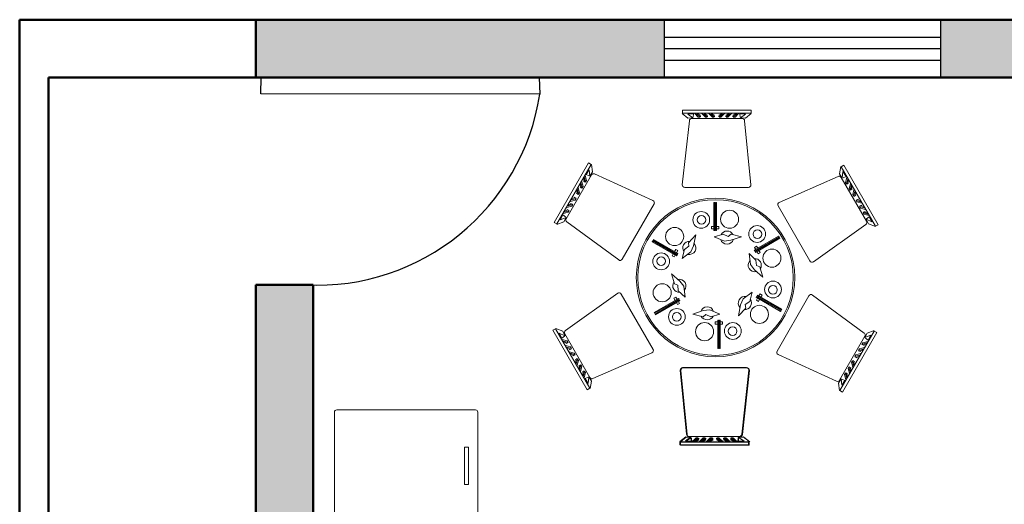
# Model space of a CAD drawing. Units: inches. Extents: x 1771 to 3025, y 319 to 889.
# Tile 32 of 35: x 2683 to 2854, y 805 to 889. Entities that reach past the tile are written whole.
import ezdxf

# ---------------------------------------------------------------- set-up
doc = ezdxf.new("R2010")
doc.units = ezdxf.units.IN
doc.header["$MEASUREMENT"] = 0
for name, color, linetype, lineweight in [('A-DOOR', 4, 'Continuous', 25), ('A-FURN', 8, 'Continuous', 18), ('A-GLAZ', 40, 'Continuous', 25), ('A-WALL', 7, 'Continuous', 50), ('A-WALL-PATT', 254, 'Continuous', 13)]:
    doc.layers.add(name, color=color, linetype=linetype, lineweight=lineweight)

# ---------------------------------------------------------------- blocks, each defined once
blk = doc.blocks.new('A$C1C317F9A')
for p, q in [((0.8756, 2.2462), (0.9155, 2.2143)), ((0.8788, 2.2685), (0.8788, 2.2478)), ((1.3449, 2.2685), (0.8788, 2.2685)), ((0.8788, 2.2478), (1.3449, 2.2478)), ((0.9139, 2.2414), (0.9522, 2.243)), ((0.949, 2.2159), (0.9139, 2.2414)), ((0.9155, 2.2143), (0.949, 2.2159)), ((0.941, 2.2111), (1.2841, 2.2111)), ((0.9522, 2.243), (0.9506, 2.2206)), ((0.9618, 2.2446), (0.9857, 2.2206)), ((0.9745, 2.243), (0.9841, 2.243)), ((0.9985, 2.2206), (0.9745, 2.243)), ((0.9841, 2.243), (0.9953, 2.2334)), ((0.9857, 2.2206), (0.9985, 2.2206)), ((0.9953, 2.2334), (0.9985, 2.2366)), ((0.9985, 2.2366), (1.0001, 2.2222)), ((1.0097, 2.2446), (1.0336, 2.2206)), ((1.0224, 2.243), (1.032, 2.243)), ((1.0464, 2.2206), (1.0224, 2.243)), ((1.032, 2.243), (1.0432, 2.2334)), ((1.0336, 2.2206), (1.0464, 2.2206)), ((1.0432, 2.2334), (1.0464, 2.2366)), ((1.0464, 2.2366), (1.048, 2.2222)), ((1.0576, 2.2446), (1.0815, 2.2206)), ((1.0703, 2.243), (1.0799, 2.243)), ((1.0943, 2.2206), (1.0703, 2.243)), ((1.0799, 2.243), (1.0911, 2.2334)), ((1.0815, 2.2206), (1.0943, 2.2206)), ((1.0911, 2.2334), (1.0943, 2.2366)), ((1.0943, 2.2366), (1.0959, 2.2222)), ((1.1262, 2.2366), (1.1246, 2.2222)), ((1.1262, 2.2206), (1.1502, 2.243)), ((1.1294, 2.2334), (1.1262, 2.2366)), ((1.139, 2.2206), (1.1262, 2.2206)), ((1.1406, 2.243), (1.1294, 2.2334)), ((1.1629, 2.2446), (1.139, 2.2206)), ((1.1502, 2.243), (1.1406, 2.243)), ((1.1741, 2.2366), (1.1725, 2.2222)), ((1.1741, 2.2206), (1.1981, 2.243)), ((1.1773, 2.2334), (1.1741, 2.2366)), ((1.1869, 2.2206), (1.1741, 2.2206)), ((1.1885, 2.243), (1.1773, 2.2334)), ((1.2108, 2.2446), (1.1869, 2.2206)), ((1.1981, 2.243), (1.1885, 2.243)), ((1.222, 2.2366), (1.2204, 2.2222)), ((1.222, 2.2206), (1.246, 2.243)), ((1.2252, 2.2334), (1.222, 2.2366)), ((1.2348, 2.2206), (1.222, 2.2206)), ((1.2364, 2.243), (1.2252, 2.2334)), ((1.2587, 2.2446), (1.2348, 2.2206)), ((1.246, 2.243), (1.2364, 2.243)), ((1.2683, 2.243), (1.2699, 2.2206)), ((1.3066, 2.2414), (1.2683, 2.243)), ((1.2715, 2.2159), (1.3066, 2.2414)), ((1.305, 2.2143), (1.2715, 2.2159)), ((1.3449, 2.2462), (1.305, 2.2143)), ((1.3449, 2.2478), (1.3449, 2.2685)), ((0.8775, 1.7628), (0.9251, 2.1968)), ((1.3, 2.1966), (1.3417, 1.7626)), ((0.2422, 1.9115), (0.0091, 1.5078)), ((0.0271, 1.4974), (0.2602, 1.9011)), ((0.2602, 1.9011), (0.2422, 1.9115)), ((0.2615, 1.9003), (0.2692, 1.8498)), ((1.9514, 1.8873), (1.9438, 1.8368)), ((1.9724, 1.8957), (1.9544, 1.8854)), ((1.9544, 1.8854), (2.1875, 1.4816)), ((2.2055, 1.492), (1.9724, 1.8957)), ((0.09, 1.5329), (0.2615, 1.8301)), ((0.2148, 1.813), (0.21, 1.8047)), ((0.21, 1.8047), (0.2127, 1.7903)), ((0.2222, 1.7811), (0.2148, 1.813)), ((0.2198, 1.8249), (0.2286, 1.7922)), ((0.2465, 1.8648), (0.226, 1.8324)), ((0.226, 1.8324), (0.2461, 1.8226)), ((0.2511, 1.8216), (0.2465, 1.8648)), ((0.2692, 1.8498), (0.2511, 1.8216)), ((0.282, 1.8367), (0.6787, 1.6557)), ((1.5338, 1.644), (1.9335, 1.8198)), ((1.9438, 1.8368), (1.9619, 1.8086)), ((1.9537, 1.8131), (2.1253, 1.516)), ((1.9619, 1.8086), (1.9665, 1.8518)), ((1.9665, 1.8518), (1.987, 1.8194)), ((1.987, 1.8194), (1.9669, 1.8096)), ((1.9932, 1.8119), (1.9844, 1.7792)), ((0.1719, 1.7419), (0.1807, 1.7092)), ((0.1888, 1.7488), (0.1844, 1.7476)), ((0.1844, 1.7476), (0.1961, 1.7391)), ((0.1909, 1.7716), (0.1861, 1.7633)), ((0.1861, 1.7633), (0.1888, 1.7488)), ((0.1982, 1.7396), (0.1909, 1.7716)), ((0.1959, 1.7834), (0.2046, 1.7507)), ((0.2046, 1.7507), (0.1982, 1.7396)), ((0.2127, 1.7903), (0.2084, 1.7891)), ((0.2084, 1.7891), (0.22, 1.7805)), ((0.2286, 1.7922), (0.2222, 1.7811)), ((1.3258, 1.7451), (0.8934, 1.7451)), ((1.9844, 1.7792), (1.9908, 1.7681)), ((1.9908, 1.7681), (1.9982, 1.8)), ((2.0046, 1.7761), (1.993, 1.7675)), ((1.9982, 1.8), (2.003, 1.7917)), ((2.003, 1.7917), (2.0003, 1.7773)), ((2.0003, 1.7773), (2.0046, 1.7761)), ((2.0171, 1.7704), (2.0084, 1.7377)), ((2.0084, 1.7377), (2.0147, 1.7266)), ((2.0147, 1.7266), (2.0221, 1.7585)), ((2.0221, 1.7585), (2.0269, 1.7502)), ((2.0269, 1.7502), (2.0242, 1.7358)), ((2.0242, 1.7358), (2.0286, 1.7346)), ((0.1583, 1.6705), (0.127, 1.6609)), ((0.127, 1.6609), (0.1318, 1.6692)), ((0.1318, 1.6692), (0.1457, 1.6741)), ((0.1445, 1.6785), (0.1577, 1.6727)), ((0.1457, 1.6741), (0.1445, 1.6785)), ((0.1519, 1.6595), (0.1583, 1.6705)), ((0.1648, 1.7073), (0.1605, 1.7061)), ((0.1605, 1.7061), (0.1721, 1.6976)), ((0.1669, 1.7301), (0.1621, 1.7218)), ((0.1621, 1.7218), (0.1648, 1.7073)), ((0.1743, 1.6982), (0.1669, 1.7301)), ((0.1807, 1.7092), (0.1743, 1.6982)), ((2.0286, 1.7346), (2.0169, 1.726)), ((2.0411, 1.7289), (2.0323, 1.6962)), ((2.0323, 1.6962), (2.0387, 1.6852)), ((2.0387, 1.6852), (2.0461, 1.7171)), ((2.0525, 1.6931), (2.0409, 1.6846)), ((2.0461, 1.7171), (2.0509, 1.7088)), ((2.0509, 1.7088), (2.0482, 1.6943)), ((2.0482, 1.6943), (2.0525, 1.6931)), ((0.0953, 1.6092), (0.128, 1.618)), ((0.1344, 1.629), (0.1031, 1.6195)), ((0.1031, 1.6195), (0.1078, 1.6278)), ((0.1078, 1.6278), (0.1217, 1.6327)), ((0.1192, 1.6507), (0.1519, 1.6595)), ((0.1217, 1.6327), (0.1206, 1.637)), ((0.1206, 1.637), (0.1338, 1.6312)), ((0.128, 1.618), (0.1344, 1.629)), ((0.6859, 1.6332), (0.4697, 1.2588)), ((1.091, 1.6437, 0.0908), (1.091, 1.4528, 0.0908)), ((1.097, 1.6437, 0.0908), (1.091, 1.6437, 0.0908)), ((1.097, 1.4528, 0.0908), (1.097, 1.6437, 0.0908)), ((1.1023, 1.6437, 0.0908), (1.1023, 1.4528, 0.0908)), ((1.1083, 1.6437, 0.0908), (1.1023, 1.6437, 0.0908)), ((1.1083, 1.4528, 0.0908), (1.1083, 1.6437, 0.0908)), ((1.7426, 1.2469), (1.5264, 1.6214)), ((2.0547, 1.6575), (2.086, 1.6479)), ((2.061, 1.6464), (2.0547, 1.6575)), ((2.0685, 1.6655), (2.0552, 1.6597)), ((2.0937, 1.6377), (2.061, 1.6464)), ((2.0673, 1.6611), (2.0685, 1.6655)), ((2.0812, 1.6562), (2.0673, 1.6611)), ((2.0786, 1.616), (2.1099, 1.6065)), ((2.085, 1.605), (2.0786, 1.616)), ((2.0924, 1.624), (2.0792, 1.6182)), ((2.086, 1.6479), (2.0812, 1.6562)), ((2.1177, 1.5962), (2.085, 1.605)), ((2.0913, 1.6196), (2.0924, 1.624)), ((2.1051, 1.6148), (2.0913, 1.6196)), ((2.1099, 1.6065), (2.1051, 1.6148)), ((0.0502, 1.5246), (0.0679, 1.5586)), ((0.0898, 1.5423), (0.0502, 1.5246)), ((0.0679, 1.5586), (0.0865, 1.5461)), ((0.0713, 1.5677), (0.104, 1.5765)), ((0.0745, 1.5125), (0.0898, 1.5423)), ((0.1104, 1.5876), (0.0791, 1.578)), ((0.0791, 1.578), (0.0839, 1.5863)), ((0.0839, 1.5863), (0.0978, 1.5912)), ((0.0966, 1.5955), (0.1098, 1.5897)), ((0.0978, 1.5912), (0.0966, 1.5955)), ((0.104, 1.5765), (0.1104, 1.5876)), ((2.1026, 1.5745), (2.1339, 1.565)), ((2.1089, 1.5635), (2.1026, 1.5745)), ((2.1164, 1.5825), (2.1031, 1.5767)), ((2.1416, 1.5547), (2.1089, 1.5635)), ((2.1152, 1.5782), (2.1164, 1.5825)), ((2.1291, 1.5733), (2.1152, 1.5782)), ((2.145, 1.5456), (2.1265, 1.5331)), ((2.1339, 1.565), (2.1291, 1.5733)), ((2.1628, 1.5116), (2.145, 1.5456)), ((0.0091, 1.5078), (0.0271, 1.4974)), ((0.0269, 1.4939), (0.0745, 1.5125)), ((0.4464, 1.2539), (0.0943, 1.5121)), ((1.0755, 1.4796, 0.0908), (1.0755, 1.4641, 0.0908)), ((1.091, 1.4796, 0.0908), (1.0755, 1.4796, 0.0908)), ((1.1023, 1.4796, 0.0908), (1.097, 1.4796, 0.0908)), ((1.125, 1.4796, 0.0908), (1.1083, 1.4796, 0.0908)), ((1.125, 1.4641, 0.0908), (1.125, 1.4796, 0.0908)), ((2.1208, 1.495), (1.7657, 1.2419)), ((2.1232, 1.5293), (2.1628, 1.5116)), ((2.1385, 1.4995), (2.1232, 1.5293)), ((2.1861, 1.4809), (2.1385, 1.4995)), ((2.1875, 1.4816), (2.2055, 1.492)), ((0.9684, 1.4231, 0.0908), (0.9184, 1.3706, 0.0908)), ((0.953, 1.3489, 0.0908), (0.9684, 1.4231, 0.0908)), ((1.0755, 1.4641, 0.0908), (1.091, 1.4641, 0.0908)), ((1.091, 1.4528, 0.0908), (1.097, 1.4528, 0.0908)), ((1.1549, 1.429, 0.0908), (1.0933, 1.4112, 0.0908)), ((1.0933, 1.4112, 0.0908), (1.1623, 1.3815, 0.0908)), ((1.097, 1.4641, 0.0908), (1.1023, 1.4641, 0.0908)), ((1.1023, 1.4528, 0.0908), (1.1083, 1.4528, 0.0908)), ((1.1083, 1.4641, 0.0908), (1.125, 1.4641, 0.0908)), ((1.1882, 1.4134, 0.0908), (1.1549, 1.429, 0.0908)), ((1.2075, 1.4282, 0.0908), (1.1882, 1.4134, 0.0908)), ((1.2061, 1.3874, 0.0908), (1.278, 1.4112, 0.0908)), ((1.278, 1.4112, 0.0908), (1.2075, 1.4282, 0.0908)), ((1.5304, 1.4154, 0.0908), (1.365, 1.3199, 0.0908)), ((1.368, 1.3147, 0.0908), (1.5334, 1.4102, 0.0908)), ((1.5361, 1.4055, 0.0908), (1.3707, 1.3101, 0.0908)), ((1.5334, 1.4102, 0.0908), (1.5304, 1.4154, 0.0908)), ((1.539, 1.4004, 0.0908), (1.5361, 1.4055, 0.0908)), ((0.6765, 1.3825, 0.0908), (0.6735, 1.3774, 0.0908)), ((0.6735, 1.3774, 0.0908), (0.8389, 1.2819, 0.0908)), ((0.8419, 1.2871, 0.0908), (0.6765, 1.3825, 0.0908)), ((0.6822, 1.3924, 0.0908), (0.6792, 1.3872, 0.0908)), ((0.6792, 1.3872, 0.0908), (0.8446, 1.2917, 0.0908)), ((0.8476, 1.2969, 0.0908), (0.6822, 1.3924, 0.0908)), ((0.9216, 1.3464, 0.0908), (0.8914, 1.3253, 0.0908)), ((0.9184, 1.3706, 0.0908), (0.9216, 1.3464, 0.0908)), ((0.9363, 1.308, 0.0908), (0.953, 1.3489, 0.0908)), ((1.1623, 1.3815, 0.0908), (1.2061, 1.3874, 0.0908)), ((1.3805, 1.3467, 0.0908), (1.3671, 1.339, 0.0908)), ((1.3671, 1.339, 0.0908), (1.3748, 1.3255, 0.0908)), ((1.3737, 1.3049, 0.0908), (1.539, 1.4004, 0.0908)), ((1.3883, 1.3333, 0.0908), (1.3805, 1.3467, 0.0908)), ((0.8156, 1.2953, 0.0908), (0.8079, 1.2819, 0.0908)), ((0.8079, 1.2819, 0.0908), (0.8213, 1.2741, 0.0908)), ((0.8213, 1.3051, 0.0908), (0.8186, 1.3005, 0.0908)), ((0.8213, 1.2741, 0.0908), (0.8291, 1.2876, 0.0908)), ((0.8327, 1.3248, 0.0908), (0.8243, 1.3103, 0.0908)), ((0.8321, 1.2927, 0.0908), (0.8348, 1.2974, 0.0908)), ((0.8461, 1.317, 0.0908), (0.8327, 1.3248, 0.0908)), ((0.8377, 1.3025, 0.0908), (0.8461, 1.317, 0.0908)), ((0.8389, 1.2819, 0.0908), (0.8419, 1.2871, 0.0908)), ((0.8446, 1.2917, 0.0908), (0.8476, 1.2969, 0.0908)), ((0.8914, 1.3253, 0.0908), (0.8761, 1.2631, 0.0908)), ((0.8761, 1.2631, 0.0908), (0.9363, 1.308, 0.0908)), ((1.3763, 1.2527, 0.0908), (1.3301, 1.2971, 0.0908)), ((1.3301, 1.2971, 0.0908), (1.3389, 1.2225, 0.0908)), ((1.365, 1.3199, 0.0908), (1.368, 1.3147, 0.0908)), ((1.3707, 1.3101, 0.0908), (1.3737, 1.3049, 0.0908)), ((1.3778, 1.3204, 0.0908), (1.3805, 1.3157, 0.0908)), ((1.3835, 1.3106, 0.0908), (1.3918, 1.2961, 0.0908)), ((1.3939, 1.3235, 0.0908), (1.3912, 1.3281, 0.0908)), ((1.3918, 1.2961, 0.0908), (1.4053, 1.3038, 0.0908)), ((1.4053, 1.3038, 0.0908), (1.3969, 1.3183, 0.0908)), ((1.3389, 1.2225, 0.0908), (1.366, 1.1876, 0.0908)), ((1.3795, 1.216, 0.0908), (1.3763, 1.2527, 0.0908)), ((1.402, 1.2067, 0.0908), (1.3795, 1.216, 0.0908)), ((1.4225, 1.1371, 0.0908), (1.402, 1.2067, 0.0908)), ((0.8033, 1.1609, 0.0908), (0.8238, 1.0913, 0.0908)), ((0.8599, 1.1105, 0.0908), (0.8033, 1.1609, 0.0908)), ((1.366, 1.1876, 0.0908), (1.4225, 1.1371, 0.0908)), ((0.8238, 1.0913, 0.0908), (0.8463, 1.0821, 0.0908)), ((0.8463, 1.0821, 0.0908), (0.8495, 1.0454, 0.0908)), ((0.8869, 1.0755, 0.0908), (0.8599, 1.1105, 0.0908)), ((0.8957, 1.0009, 0.0908), (0.8869, 1.0755, 0.0908)), ((0.0847, 0.7751), (0.4398, 1.0281)), ((0.4628, 1.0231), (0.679, 0.6486)), ((0.834, 1.0019, 0.0908), (0.8206, 0.9942, 0.0908)), ((0.8424, 0.9875, 0.0908), (0.834, 1.0019, 0.0908)), ((0.8495, 1.0454, 0.0908), (0.8957, 1.0009, 0.0908)), ((1.3498, 1.0349, 0.0908), (1.2896, 0.99, 0.0908)), ((1.3344, 0.9727, 0.0908), (1.3498, 1.0349, 0.0908)), ((1.3813, 1.0063, 0.0908), (1.3783, 1.0011, 0.0908)), ((1.3783, 1.0011, 0.0908), (1.5437, 0.9057, 0.0908)), ((1.5466, 0.9108, 0.0908), (1.3813, 1.0063, 0.0908)), ((1.3869, 1.0161, 0.0908), (1.384, 1.011, 0.0908)), ((1.384, 1.011, 0.0908), (1.5493, 0.9155, 0.0908)), ((1.5523, 0.9207, 0.0908), (1.3869, 1.0161, 0.0908)), ((1.3938, 1.0053, 0.0908), (1.3911, 1.0006, 0.0908)), ((1.4045, 1.0239, 0.0908), (1.3968, 1.0105, 0.0908)), ((1.418, 1.0162, 0.0908), (1.4045, 1.0239, 0.0908)), ((1.4102, 1.0027, 0.0908), (1.418, 1.0162, 0.0908)), ((1.5196, 0.6368), (1.7358, 1.0113)), ((1.7591, 1.0162), (2.1111, 0.7579)), ((0.8522, 0.9931, 0.0908), (0.6868, 0.8977, 0.0908)), ((0.6898, 0.8925, 0.0908), (0.8552, 0.988, 0.0908)), ((0.8578, 0.9833, 0.0908), (0.6925, 0.8878, 0.0908)), ((0.6955, 0.8827, 0.0908), (0.8608, 0.9781, 0.0908)), ((0.8206, 0.9942, 0.0908), (0.8289, 0.9797, 0.0908)), ((0.8319, 0.9745, 0.0908), (0.8346, 0.9699, 0.0908)), ((0.8376, 0.9647, 0.0908), (0.8453, 0.9513, 0.0908)), ((0.848, 0.9776, 0.0908), (0.8453, 0.9823, 0.0908)), ((0.8453, 0.9513, 0.0908), (0.8588, 0.959, 0.0908)), ((0.8588, 0.959, 0.0908), (0.851, 0.9725, 0.0908)), ((0.8552, 0.988, 0.0908), (0.8522, 0.9931, 0.0908)), ((0.8608, 0.9781, 0.0908), (0.8578, 0.9833, 0.0908)), ((1.2728, 0.9491, 0.0908), (1.2574, 0.875, 0.0908)), ((1.2896, 0.99, 0.0908), (1.2728, 0.9491, 0.0908)), ((1.3042, 0.9516, 0.0908), (1.3344, 0.9727, 0.0908)), ((1.3074, 0.9275, 0.0908), (1.3042, 0.9516, 0.0908)), ((1.3881, 0.9955, 0.0908), (1.3797, 0.981, 0.0908)), ((1.3797, 0.981, 0.0908), (1.3932, 0.9732, 0.0908)), ((1.3932, 0.9732, 0.0908), (1.4015, 0.9877, 0.0908)), ((1.4045, 0.9929, 0.0908), (1.4072, 0.9975, 0.0908)), ((0.6868, 0.8977, 0.0908), (0.6898, 0.8925, 0.0908)), ((0.6925, 0.8878, 0.0908), (0.6955, 0.8827, 0.0908)), ((1.0198, 0.9106, 0.0908), (0.9478, 0.8869, 0.0908)), ((0.9478, 0.8869, 0.0908), (1.0183, 0.8698, 0.0908)), ((1.0183, 0.8698, 0.0908), (1.0376, 0.8846, 0.0908)), ((1.0636, 0.9165, 0.0908), (1.0198, 0.9106, 0.0908)), ((1.0376, 0.8846, 0.0908), (1.071, 0.8691, 0.0908)), ((1.1326, 0.8869, 0.0908), (1.0636, 0.9165, 0.0908)), ((1.071, 0.8691, 0.0908), (1.1326, 0.8869, 0.0908)), ((1.2574, 0.875, 0.0908), (1.3074, 0.9275, 0.0908)), ((1.5437, 0.9057, 0.0908), (1.5466, 0.9108, 0.0908)), ((1.5493, 0.9155, 0.0908), (1.5523, 0.9207, 0.0908)), ((1.1175, 0.8339, 0.0908), (1.1008, 0.8339, 0.0908)), ((1.1008, 0.8339, 0.0908), (1.1008, 0.8184, 0.0908)), ((1.1008, 0.8184, 0.0908), (1.1175, 0.8184, 0.0908)), ((1.1235, 0.8453, 0.0908), (1.1175, 0.8453, 0.0908)), ((1.1175, 0.8453, 0.0908), (1.1175, 0.6543, 0.0908)), ((1.1235, 0.6543, 0.0908), (1.1235, 0.8453, 0.0908)), ((1.1289, 0.8339, 0.0908), (1.1235, 0.8339, 0.0908)), ((1.1235, 0.8184, 0.0908), (1.1289, 0.8184, 0.0908)), ((1.1349, 0.8453, 0.0908), (1.1289, 0.8453, 0.0908)), ((1.1289, 0.8453, 0.0908), (1.1289, 0.6543, 0.0908)), ((1.1349, 0.6543, 0.0908), (1.1349, 0.8453, 0.0908)), ((1.1504, 0.8339, 0.0908), (1.1349, 0.8339, 0.0908)), ((1.1349, 0.8184, 0.0908), (1.1504, 0.8184, 0.0908)), ((1.1504, 0.8184, 0.0908), (1.1504, 0.8339, 0.0908)), ((0.018, 0.7884), (0, 0.778)), ((0, 0.778), (0.2331, 0.3743)), ((0.2511, 0.3847), (0.018, 0.7884)), ((0.0193, 0.7892), (0.0669, 0.7706)), ((0.0427, 0.7584), (0.0604, 0.7244)), ((0.0823, 0.7407), (0.0427, 0.7584)), ((0.0604, 0.7244), (0.079, 0.737)), ((0.0669, 0.7706), (0.0823, 0.7407)), ((0.2517, 0.4569), (0.0802, 0.7541)), ((2.1155, 0.7371), (1.9439, 0.4399)), ((2.1784, 0.7726), (1.9453, 0.3689)), ((1.9633, 0.3585), (2.1964, 0.7622)), ((2.131, 0.7576), (2.1156, 0.7277)), ((2.1156, 0.7277), (2.1553, 0.7454)), ((2.1786, 0.7762), (2.131, 0.7576)), ((2.1553, 0.7454), (2.1375, 0.7114)), ((2.1964, 0.7622), (2.1784, 0.7726)), ((0.0638, 0.7153), (0.0965, 0.7066)), ((0.0716, 0.7051), (0.0764, 0.6968)), ((0.1029, 0.6955), (0.0716, 0.7051)), ((0.0764, 0.6968), (0.0903, 0.6919)), ((0.0878, 0.6738), (0.1205, 0.6651)), ((0.0891, 0.6875), (0.1023, 0.6933)), ((0.0903, 0.6919), (0.0891, 0.6875)), ((0.0965, 0.7066), (0.1029, 0.6955)), ((2.1014, 0.6935), (2.095, 0.6825)), ((2.095, 0.6825), (2.1264, 0.6921)), ((2.1089, 0.6745), (2.0956, 0.6803)), ((2.1341, 0.7023), (2.1014, 0.6935)), ((2.1216, 0.6838), (2.1077, 0.6789)), ((2.1077, 0.6789), (2.1089, 0.6745)), ((2.1375, 0.7114), (2.119, 0.724)), ((2.1264, 0.6921), (2.1216, 0.6838)), ((0.0955, 0.6636), (0.1003, 0.6553)), ((0.1269, 0.654), (0.0955, 0.6636)), ((0.1003, 0.6553), (0.1142, 0.6504)), ((0.1117, 0.6324), (0.1444, 0.6236)), ((0.1131, 0.646), (0.1263, 0.6518)), ((0.1142, 0.6504), (0.1131, 0.646)), ((0.1195, 0.6221), (0.1243, 0.6138)), ((0.1508, 0.6125), (0.1195, 0.6221)), ((0.1205, 0.6651), (0.1269, 0.654)), ((0.1243, 0.6138), (0.1382, 0.6089)), ((0.137, 0.6046), (0.1502, 0.6104)), ((0.1382, 0.6089), (0.137, 0.6046)), ((0.1444, 0.6236), (0.1508, 0.6125)), ((0.6716, 0.6261), (0.272, 0.4503)), ((1.1175, 0.6543, 0.0908), (1.1235, 0.6543, 0.0908)), ((1.1289, 0.6543, 0.0908), (1.1349, 0.6543, 0.0908)), ((1.9235, 0.4334), (1.5268, 0.6143)), ((2.0535, 0.6106), (2.0471, 0.5995)), ((2.0471, 0.5995), (2.0785, 0.6091)), ((2.0862, 0.6194), (2.0535, 0.6106)), ((2.0737, 0.6008), (2.0598, 0.5959)), ((2.0775, 0.6521), (2.0711, 0.641)), ((2.0711, 0.641), (2.1024, 0.6506)), ((2.0849, 0.633), (2.0717, 0.6388)), ((2.0785, 0.6091), (2.0737, 0.6008)), ((2.1102, 0.6608), (2.0775, 0.6521)), ((2.0976, 0.6423), (2.0837, 0.6374)), ((2.0837, 0.6374), (2.0849, 0.633)), ((2.1024, 0.6506), (2.0976, 0.6423)), ((0.153, 0.5769), (0.1646, 0.5855)), ((0.1573, 0.5757), (0.153, 0.5769)), ((0.1546, 0.5613), (0.1573, 0.5757)), ((0.1594, 0.553), (0.1546, 0.5613)), ((0.1668, 0.5849), (0.1594, 0.553)), ((0.1644, 0.5411), (0.1732, 0.5738)), ((0.1732, 0.5738), (0.1668, 0.5849)), ((0.1769, 0.5354), (0.1885, 0.544)), ((0.1813, 0.5343), (0.1769, 0.5354)), ((0.1786, 0.5198), (0.1813, 0.5343)), ((0.1907, 0.5434), (0.1834, 0.5115)), ((0.1971, 0.5323), (0.1907, 0.5434)), ((2.0248, 0.5608), (2.0312, 0.5719)), ((2.0336, 0.5281), (2.0248, 0.5608)), ((2.0312, 0.5719), (2.0386, 0.54)), ((2.045, 0.5639), (2.0334, 0.5725)), ((2.0386, 0.54), (2.0433, 0.5483)), ((2.0406, 0.5627), (2.045, 0.5639)), ((2.0433, 0.5483), (2.0406, 0.5627)), ((2.061, 0.5915), (2.0477, 0.5973)), ((2.0598, 0.5959), (2.061, 0.5915)), ((0.1834, 0.5115), (0.1786, 0.5198)), ((0.1884, 0.4996), (0.1971, 0.5323)), ((0.2009, 0.4939), (0.2125, 0.5025)), ((0.2052, 0.4928), (0.2009, 0.4939)), ((0.2025, 0.4783), (0.2052, 0.4928)), ((0.2073, 0.47), (0.2025, 0.4783)), ((0.2147, 0.5019), (0.2073, 0.47)), ((0.2123, 0.4582), (0.2211, 0.4909)), ((0.2211, 0.4909), (0.2147, 0.5019)), ((0.9055, 0.0734), (0.8638, 0.5074)), ((0.9096, 0.0719), (0.8679, 0.5059)), ((0.8797, 0.5249), (1.3121, 0.5249)), ((0.8838, 0.5234), (1.3162, 0.5234)), ((1.328, 0.5072), (1.2804, 0.0732)), ((1.3321, 0.5057), (1.2845, 0.0717)), ((1.9769, 0.4779), (1.9833, 0.4889)), ((1.9857, 0.4451), (1.9769, 0.4779)), ((1.9833, 0.4889), (1.9907, 0.457)), ((1.9971, 0.4809), (1.9855, 0.4895)), ((1.9927, 0.4798), (1.9971, 0.4809)), ((1.9955, 0.4653), (1.9927, 0.4798)), ((2.0009, 0.5193), (2.0072, 0.5304)), ((2.0096, 0.4866), (2.0009, 0.5193)), ((2.0072, 0.5304), (2.0146, 0.4985)), ((2.0211, 0.5224), (2.0094, 0.531)), ((2.0146, 0.4985), (2.0194, 0.5068)), ((2.0167, 0.5212), (2.0211, 0.5224)), ((2.0194, 0.5068), (2.0167, 0.5212)), ((0.2185, 0.4507), (0.2386, 0.4604)), ((0.239, 0.4183), (0.2185, 0.4507)), ((0.2436, 0.4615), (0.239, 0.4183)), ((0.2617, 0.4332), (0.2436, 0.4615)), ((0.254, 0.3827), (0.2617, 0.4332)), ((1.9363, 0.4202), (1.9544, 0.4484)), ((1.9439, 0.3697), (1.9363, 0.4202)), ((1.9544, 0.4484), (1.9589, 0.4053)), ((1.9589, 0.4053), (1.9795, 0.4377)), ((1.9795, 0.4377), (1.9593, 0.4474)), ((1.9907, 0.457), (1.9955, 0.4653)), ((0.2331, 0.3743), (0.2511, 0.3847)), ((1.9453, 0.3689), (1.9633, 0.3585)), ((0.8605, 0.0239), (0.9005, 0.0558)), ((0.8605, 0.0223), (0.8605, 0.0015)), ((1.3267, 0.0223), (0.8605, 0.0223)), ((0.8605, 0.0015), (1.3267, 0.0015)), ((0.8647, 0.0223), (0.9046, 0.0543)), ((0.8647, 0.0207), (0.8647, 0)), ((1.3308, 0.0207), (0.8647, 0.0207)), ((0.8647, 0), (1.3308, 0)), ((0.934, 0.0542), (0.8989, 0.0286)), ((0.8989, 0.0286), (0.9372, 0.027)), ((0.9005, 0.0558), (0.934, 0.0542)), ((0.9381, 0.0527), (0.903, 0.0271)), ((0.903, 0.0271), (0.9413, 0.0255)), ((0.9046, 0.0543), (0.9381, 0.0527)), ((1.2645, 0.059), (0.9213, 0.059)), ((1.2686, 0.0574), (0.9255, 0.0574)), ((0.9372, 0.027), (0.9356, 0.0494)), ((0.9413, 0.0255), (0.9397, 0.0479)), ((0.9468, 0.0255), (0.9707, 0.0494)), ((0.9509, 0.0239), (0.9748, 0.0479)), ((0.9835, 0.0494), (0.9595, 0.027)), ((0.9595, 0.027), (0.9691, 0.027)), ((0.9876, 0.0479), (0.9636, 0.0255)), ((0.9636, 0.0255), (0.9732, 0.0255)), ((0.9691, 0.027), (0.9803, 0.0366)), ((0.9707, 0.0494), (0.9835, 0.0494)), ((0.9732, 0.0255), (0.9844, 0.0351)), ((0.9748, 0.0479), (0.9876, 0.0479)), ((0.9803, 0.0366), (0.9835, 0.0334)), ((0.9835, 0.0334), (0.9851, 0.0478)), ((0.9844, 0.0351), (0.9876, 0.0319)), ((0.9876, 0.0319), (0.9892, 0.0463)), ((0.9946, 0.0255), (1.0186, 0.0494)), ((0.9988, 0.0239), (1.0227, 0.0479)), ((1.0314, 0.0494), (1.0074, 0.027)), ((1.0074, 0.027), (1.017, 0.027)), ((1.0355, 0.0479), (1.0115, 0.0255)), ((1.0115, 0.0255), (1.0211, 0.0255)), ((1.017, 0.027), (1.0282, 0.0366)), ((1.0186, 0.0494), (1.0314, 0.0494)), ((1.0211, 0.0255), (1.0323, 0.0351)), ((1.0227, 0.0479), (1.0355, 0.0479)), ((1.0282, 0.0366), (1.0314, 0.0334)), ((1.0314, 0.0334), (1.033, 0.0478)), ((1.0323, 0.0351), (1.0355, 0.0319)), ((1.0355, 0.0319), (1.0371, 0.0463)), ((1.0425, 0.0255), (1.0665, 0.0494)), ((1.0467, 0.0239), (1.0706, 0.0479)), ((1.0793, 0.0494), (1.0553, 0.027)), ((1.0553, 0.027), (1.0649, 0.027)), ((1.0834, 0.0479), (1.0594, 0.0255)), ((1.0594, 0.0255), (1.069, 0.0255)), ((1.0649, 0.027), (1.0761, 0.0366)), ((1.0665, 0.0494), (1.0793, 0.0494)), ((1.069, 0.0255), (1.0802, 0.0351)), ((1.0706, 0.0479), (1.0834, 0.0479)), ((1.0761, 0.0366), (1.0793, 0.0334)), ((1.0793, 0.0334), (1.0809, 0.0478)), ((1.0802, 0.0351), (1.0834, 0.0319)), ((1.0834, 0.0319), (1.085, 0.0463)), ((1.1112, 0.0334), (1.1096, 0.0478)), ((1.1112, 0.0494), (1.1351, 0.027)), ((1.124, 0.0494), (1.1112, 0.0494)), ((1.1144, 0.0366), (1.1112, 0.0334)), ((1.1153, 0.0319), (1.1137, 0.0463)), ((1.1256, 0.027), (1.1144, 0.0366)), ((1.1153, 0.0479), (1.1393, 0.0255)), ((1.1281, 0.0479), (1.1153, 0.0479)), ((1.1185, 0.0351), (1.1153, 0.0319)), ((1.1297, 0.0255), (1.1185, 0.0351)), ((1.1479, 0.0255), (1.124, 0.0494)), ((1.1351, 0.027), (1.1256, 0.027)), ((1.152, 0.0239), (1.1281, 0.0479)), ((1.1393, 0.0255), (1.1297, 0.0255)), ((1.1591, 0.0334), (1.1575, 0.0478)), ((1.1591, 0.0494), (1.183, 0.027)), ((1.1719, 0.0494), (1.1591, 0.0494)), ((1.1623, 0.0366), (1.1591, 0.0334)), ((1.1632, 0.0319), (1.1616, 0.0463)), ((1.1735, 0.027), (1.1623, 0.0366)), ((1.1632, 0.0479), (1.1872, 0.0255)), ((1.176, 0.0479), (1.1632, 0.0479)), ((1.1664, 0.0351), (1.1632, 0.0319)), ((1.1776, 0.0255), (1.1664, 0.0351)), ((1.1958, 0.0255), (1.1719, 0.0494)), ((1.183, 0.027), (1.1735, 0.027)), ((1.1999, 0.0239), (1.176, 0.0479)), ((1.1872, 0.0255), (1.1776, 0.0255)), ((1.207, 0.0334), (1.2054, 0.0478)), ((1.207, 0.0494), (1.2309, 0.027)), ((1.2198, 0.0494), (1.207, 0.0494)), ((1.2102, 0.0366), (1.207, 0.0334)), ((1.2111, 0.0319), (1.2095, 0.0463)), ((1.2214, 0.027), (1.2102, 0.0366)), ((1.2111, 0.0479), (1.235, 0.0255)), ((1.2239, 0.0479), (1.2111, 0.0479)), ((1.2143, 0.0351), (1.2111, 0.0319)), ((1.2255, 0.0255), (1.2143, 0.0351)), ((1.2437, 0.0255), (1.2198, 0.0494)), ((1.2309, 0.027), (1.2214, 0.027)), ((1.2478, 0.0239), (1.2239, 0.0479)), ((1.235, 0.0255), (1.2255, 0.0255)), ((1.2533, 0.027), (1.2549, 0.0494)), ((1.2916, 0.0286), (1.2533, 0.027)), ((1.29, 0.0558), (1.2565, 0.0542)), ((1.2565, 0.0542), (1.2916, 0.0286)), ((1.2574, 0.0255), (1.259, 0.0479)), ((1.2957, 0.0271), (1.2574, 0.0255)), ((1.2941, 0.0543), (1.2606, 0.0527)), ((1.2606, 0.0527), (1.2957, 0.0271)), ((1.3299, 0.0239), (1.29, 0.0558)), ((1.334, 0.0223), (1.2941, 0.0543)), ((1.3267, 0.0015), (1.3267, 0.0223)), ((1.3308, 0), (1.3308, 0.0207))]:
    blk.add_line(p, q)
for centre, radius in [((1.1027, 1.135), 0.537), ((1.1027, 1.135), 0.527), ((1.0059, 1.525, 0.0908), 0.0569), ((1.0072, 1.5257, 0.0908), 0.0294), ((1.1975, 1.5297, 0.0908), 0.0613), ((0.8256, 1.4126, 0.0908), 0.0613), ((1.385, 1.4297, 0.0908), 0.0569), ((1.3863, 1.4289, 0.0908), 0.0294), ((0.7338, 1.2443, 0.0908), 0.0569), ((0.7339, 1.2458, 0.0908), 0.0294), ((1.4849, 1.2661, 0.0908), 0.0613), ((0.741, 1.0319, 0.0908), 0.0613), ((1.4921, 1.0537, 0.0908), 0.0569), ((1.492, 1.0522, 0.0908), 0.0294), ((1.4003, 0.8854, 0.0908), 0.0613), ((0.8408, 0.8683, 0.0908), 0.0569), ((0.8396, 0.8691, 0.0908), 0.0294), ((1.0283, 0.7683, 0.0908), 0.0613), ((1.2199, 0.773, 0.0908), 0.0569), ((1.2186, 0.7723, 0.0908), 0.0294)]:
    blk.add_circle(centre, radius)
for centre, radius, start, end in [((0.941, 2.1951), 0.016, 90, 173.74283), ((1.2841, 2.1951), 0.016, 5.48012, 90), ((0.2754, 1.8222), 0.016, 65.48012, 150), ((1.9399, 1.8052), 0.016, 30, 113.74283), ((0.8934, 1.7611), 0.016, 173.74283, 270), ((1.3258, 1.7611), 0.016, 270, 5.48012), ((0.6721, 1.6412), 0.016, 330, 65.48012), ((1.5403, 1.6294), 0.016, 113.74283, 210), ((0.1038, 1.525), 0.016, 150, 233.74283), ((2.1115, 1.508), 0.016, 305.48012, 30), ((1.1801, 1.4052, 0.0908), 0.0446, 26.66413, 154.14416), ((0.9246, 1.3353, 0.0908), 0.0446, 86.66413, 214.14416), ((0.9246, 1.3353, 0.0908), 0.0446, 257.0611, 44.06617), ((1.1801, 1.4052, 0.0908), 0.0446, 197.0611, 344.06617), ((0.4559, 1.2667), 0.016, 233.74283, 330), ((1.3684, 1.2189, 0.0908), 0.0446, 137.0611, 284.06617), ((1.3684, 1.2189, 0.0908), 0.0446, 326.66413, 94.14416), ((1.7565, 1.2549), 0.016, 210, 305.48012), ((0.8574, 1.0791, 0.0908), 0.0446, 146.66413, 274.14416), ((0.8574, 1.0791, 0.0908), 0.0446, 317.0611, 104.06617), ((0.449, 1.0151), 0.016, 30, 125.48012), ((1.3012, 0.9627, 0.0908), 0.0446, 77.0611, 224.06617), ((1.7496, 1.0033), 0.016, 53.74283, 150), ((1.0457, 0.8928, 0.0908), 0.0446, 17.0611, 164.06617), ((1.3012, 0.9627, 0.0908), 0.0446, 266.66413, 34.14416), ((1.0457, 0.8928, 0.0908), 0.0446, 206.66413, 334.14416), ((0.094, 0.7621), 0.016, 125.48012, 210), ((2.1017, 0.7451), 0.016, 330, 53.74283), ((0.6652, 0.6407), 0.016, 293.74283, 30), ((1.5334, 0.6288), 0.016, 150, 245.48012), ((0.8797, 0.5089), 0.016, 90, 185.48012), ((0.8838, 0.5074), 0.016, 90, 185.48012), ((1.3121, 0.5089), 0.016, 353.74283, 90), ((1.3162, 0.5074), 0.016, 353.74283, 90), ((0.2656, 0.4649), 0.016, 210, 293.74283), ((1.9301, 0.4479), 0.016, 245.48012, 330), ((0.9213, 0.0749), 0.016, 185.48012, 270), ((0.9255, 0.0734), 0.016, 185.48012, 270), ((1.2645, 0.0749), 0.016, 270, 353.74283), ((1.2686, 0.0734), 0.016, 270, 353.74283)]:
    blk.add_arc(centre, radius, start, end)
blk = doc.blocks.new('A$C43BC2F3A')
for p, q in [((0, 1490.5), (0, 93.5)), ((10, 1500), (590, 1500)), ((600, 1490), (600, 93.5)), ((590, 83.5), (10.3, 83.5)), ((22.6, 83.5), (561, 83.5)), ((30.8, 0), (30.8, 83.5)), ((561, 83.5), (561, 0)), ((561, 0), (30.8, 0))]:
    blk.add_line(p, q)
for points in [[(561, 1344.2), (561, 1188.3), (544.3, 1188.3), (544.3, 1344.2)], [(561, 949), (561, 743), (544.3, 743), (544.3, 949)]]:
    blk.add_lwpolyline(points, close=True)
for points in [[(600, 1060.3), (0, 1060.3)], [(600, 1043.6), (0, 1043.6)]]:
    blk.add_lwpolyline(points)
for centre, radius, start, end in [((10, 1490), 10, 90, 180), ((590, 1490), 10, 0, 90), ((10.5, 94), 10.5, 182.8791, 268.8051), ((590, 93.5), 10, 270, 0)]:
    blk.add_arc(centre, radius, start, end)
blk = doc.blocks.new('DOOR-39')
blk.add_lwpolyline([(48.33, 36.05), (48.44, 33.13), (0, 33.22), (0.05, 36.05)], close=True)
blk.add_arc((9.8, 39.1), 39.1, 267.0753, 351.2184)
blk = doc.blocks.new('WIN-48')
for p, q in [((0, 0), (0, 10)), ((48, 0), (48, 10)), ((0, 7), (48, 7)), ((0, 5), (48, 5)), ((0, 3), (48, 3))]:
    blk.add_line(p, q)

msp = doc.modelspace()

# ---------------------------------------------------------------- hatches: boundary and pattern name
at = {"layer": 'A-WALL-PATT'}
h = msp.add_hatch(color=256, dxfattribs=at)
h.dxf.hatch_style = 1
h.paths.add_polyline_path([(2870.68, 879.48), (2892.73, 879.48), (2892.73, 889.48), (2842.68, 889.48), (2842.68, 879.48), (2865.68, 879.48), (2865.68, 831.48), (2870.68, 831.48)])
h.paths.add_polyline_path([(2983.64, 889.48), (2940.73, 889.48), (2940.73, 879.48), (2961.68, 879.48), (2961.68, 795.48), (2865.68, 795.48), (2865.68, 759.48), (2865.68, 665.48), (2870.68, 665.48), (2870.68, 712.85), (2870.68, 790.48), (2978.68, 790.48), (2978.68, 795.48), (2966.68, 795.48), (2966.68, 879.48), (2983.64, 879.48)])
h.paths.add_polyline_path([(3024.68, 889.48), (3001.64, 889.48), (3001.64, 879.48), (3014.68, 879.48), (3014.68, 790.48), (3014.68, 769.46), (3024.68, 769.46)])
h.paths.add_polyline_path([(3024.68, 721.46), (3014.68, 721.46), (3014.68, 670.48), (2906.68, 670.48), (2906.68, 665.48), (2925.68, 665.48), (2925.68, 653.48), (2930.68, 653.48), (2930.68, 665.48), (3014.68, 665.48), (3014.68, 650.02), (3024.68, 650.02)])
h.paths.add_polyline_path([(3024.68, 632.02), (3014.68, 632.02), (3014.68, 617.48), (2925.68, 617.48), (2906.68, 617.48), (2906.68, 612.48), (3014.68, 612.48), (3014.68, 581.96), (3024.68, 581.96)])
h.paths.add_polyline_path([(3024.68, 533.96), (3014.68, 533.96), (3014.68, 480.48), (2870.68, 480.48), (2870.68, 617.48), (2860.68, 617.48), (2860.68, 544.48), (2769.68, 544.48), (2769.68, 534.48), (2860.68, 534.48), (2860.68, 470.48), (3014.68, 470.48), (3014.68, 453.61), (3024.68, 453.61)])
h.paths.add_polyline_path([(3024.68, 405.61), (3014.68, 405.61), (3014.68, 394.48), (2860.68, 394.48), (2860.68, 384.48), (3024.68, 384.48)])
h.paths.add_polyline_path([(2733.68, 643.43), (2723.68, 643.43), (2723.68, 534.48), (2733.68, 534.48)])
h.paths.add_polyline_path([(2733.68, 754.48), (2829.68, 754.48), (2829.68, 759.48), (2733.68, 759.48), (2733.68, 843.44, -0.008336), (2732.38, 843.48), (2723.68, 843.48), (2723.68, 691.43), (2733.68, 691.43)])
h.paths.add_polyline_path([(2794.68, 889.48), (2723.68, 889.48), (2723.68, 879.48), (2794.68, 879.48)])

# ---------------------------------------------------------------- linework, layer by layer
at = {"layer": 'A-WALL'}
for p, q in [((3024.68, 889.48), (2682.68, 889.48)), ((2682.68, 889.48), (2682.68, 534.48)), ((2723.68, 889.48), (2723.68, 879.48)), ((2865.68, 879.48), (2687.68, 879.48)), ((2687.68, 879.48), (2687.68, 534.48)), ((2733.68, 843.48), (2723.68, 843.48)), ((2723.68, 843.48), (2723.68, 534.48)), ((2733.68, 843.48), (2733.68, 759.48))]:
    msp.add_line(p, q, dxfattribs=at)

# ---------------------------------------------------------------- block references
at = {"layer": 'A-DOOR'}
msp.add_blockref('DOOR-39', (2724.57, 843.43), dxfattribs=at)
at = {"layer": 'A-FURN'}
for name, p, xscale, yscale, zscale in [('A$C1C317F9A', (2775.28, 815.67), 25.6235517785217, 25.6235517785217, 25.6235517785217), ('A$C43BC2F3A', (2737.33, 759.48), 0.0415387277892195, 0.0415387277892195, 0.0415387277892195)]:
    msp.add_blockref(name, p, dxfattribs=dict(at, xscale=xscale, yscale=yscale, zscale=zscale))
at = {"layer": 'A-GLAZ'}
msp.add_blockref('WIN-48', (2794.68, 879.48), dxfattribs=at)

doc.saveas('drawing.dxf')
